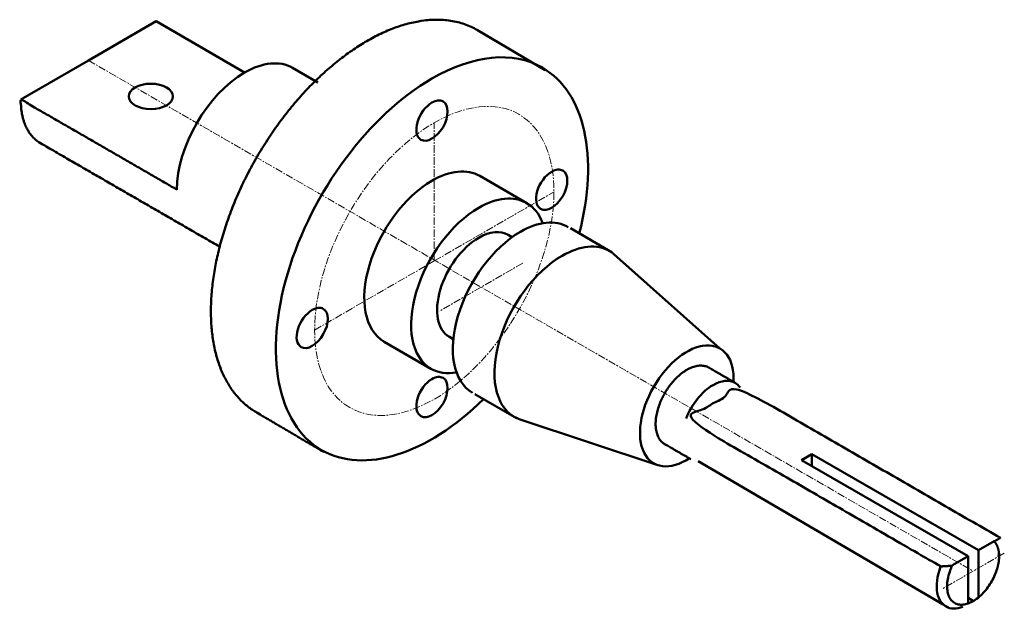
# Model space of a CAD drawing. Units: millimetres. Extents: x -23 to 141, y -9 to 89.
import ezdxf

# ---------------------------------------------------------------- set-up
doc = ezdxf.new("R2010")
doc.units = ezdxf.units.MM
doc.header["$MEASUREMENT"] = 0
doc.linetypes.add('CENTER', pattern=[2, 1.25, -0.25, 0.25, -0.25])
doc.layers.add('M-CNTR', color=4, linetype='CENTER', lineweight=18)
doc.layers.add('M-OUTL', color=7, linetype='Continuous', lineweight=50)

msp = doc.modelspace()

# ---------------------------------------------------------------- linework, layer by layer
at = {"layer": 'M-CNTR'}
for p, q in [((-11.24, 81.97), (135.98, -3.03)), ((46.33, 48.59), (46.33, 71.59)), ((61.05, 48.23), (47.19, 40.23)), ((141.18, -0.03), (130.79, -6.03))]:
    msp.add_line(p, q, dxfattribs=at)
msp.add_lwpolyline([(26.41, 37.09), (46.33, 48.59), (66.25, 60.09)], dxfattribs=at)
msp.add_ellipse((46.33, 48.59), major_axis=(-14.08, -24.4), ratio=0.57735, dxfattribs=at)
at = {"layer": 'M-OUTL'}
for p, q in [((53.5, 87.01), (64.8, 80.35)), ((26.95, 78.28), (22.72, 80.73)), ((61.7, 58.23), (53.9, 62.73)), ((59.29, 52.54), (58.63, 52.92)), ((69.01, 54.02), (75.94, 50.02)), ((75.72, 50.14), (93.86, 34.01)), ((45.77, 30.65), (37.98, 35.15)), ((49.49, 35.57), (48.84, 35.95)), ((53.09, 26.44), (60.02, 22.44)), ((83.55, 14.58), (60.62, 22.2)), ((109.16, 16.44), (107.43, 15.44)), ((136.87, 0.44), (109.16, 16.44)), ((109.16, 14.44), (109.16, 16.44)), ((90.25, 15.26), (131.02, -8.58)), ((135.14, -0.56), (107.43, 15.44)), ((136.87, 0.44), (139.47, 1.94)), ((136.87, 0.44), (136.87, -7.46)), ((132.54, -2.06), (135.14, -0.56)), ((135.14, -0.56), (135.14, -8.46)), ((136.01, -7.98), (135.14, -7.48))]:
    msp.add_line(p, q, dxfattribs=at)
msp.add_lwpolyline([(-22.5, 75.47), (-11.24, 81.97), (0.02, 88.47), (14.74, 79.97)], dxfattribs=at)
for centre, major_axis, start_param, end_param in [((45.94, 48.94), (18.37, 31.82), 0, 0.785398), ((14.76, 66.94), (7.96, 13.79), 0, 0.785398), ((45.94, 48.94), (18.37, 31.82), 5.160577, 6.283185), ((14.76, 66.94), (7.96, 13.79), 0.785398, 2.356194), ((45.94, 48.94), (18.37, 31.82), 0.785398, 3.141593), ((45.94, 71.94), (1.84, 3.18), 0, 0.785398), ((45.94, 71.94), (1.84, 3.18), 0.785398, 3.141593), ((45.94, 71.94), (1.84, 3.18), 3.141593, 6.283185), ((45.94, 48.94), (7.96, 13.79), 0, 0.785398), ((65.86, 60.44), (1.84, 3.18), 0, 0.785398), ((65.86, 60.44), (1.84, 3.18), 0.785398, 3.141593), ((65.86, 60.44), (1.84, 3.18), 3.141593, 6.283185), ((45.94, 48.94), (7.96, 13.79), 0.785398, 3.141593), ((53.73, 44.44), (7.96, 13.79), 0, 0.785398), ((53.73, 44.44), (7.96, 13.79), 0.785398, 3.141593), ((53.73, 44.44), (7.96, 13.79), 5.832989, 6.283185), ((60.66, 40.44), (7.96, 13.79), 0, 0.785398), ((53.73, 44.44), (4.9, 8.49), 0.785398, 3.141593), ((60.66, 40.44), (7.96, 13.79), 0.785398, 3.141593), ((53.73, 44.44), (4.9, 8.49), 0, 0.785398), ((67.59, 36.44), (7.96, 13.79), 0, 0.785398), ((67.59, 36.44), (7.96, 13.79), 0.785398, 3.141593), ((26.02, 37.44), (1.84, 3.18), 0.785398, 3.141593), ((26.02, 37.44), (1.84, 3.18), 3.141593, 6.283185), ((26.02, 37.44), (1.84, 3.18), 0, 0.785398), ((88.35, 24.47), (-5.51, -9.55), 2.298971, 7.125807), ((53.73, 44.44), (7.96, 13.79), 3.141593, 3.591789), ((45.94, 25.94), (1.84, 3.18), 0.785398, 3.141593), ((45.94, 25.94), (1.84, 3.18), 3.141593, 6.283185), ((45.94, 25.94), (1.84, 3.18), 0, 0.785398), ((92.71, 21.94), (3.67, 6.36), 0.785398, 1.832596), ((92.71, 21.94), (3.67, 6.36), 0, 0.785398), ((92.71, 21.94), (3.67, 6.36), 6.021386, 6.283185), ((45.94, 48.94), (18.37, 31.82), 3.141593, 4.264201), ((67.59, 36.44), (7.96, 13.79), 3.141593, 3.259718), ((135.12, -2.53), (-3.67, -6.36), 8.471932, 8.552132), ((135.12, -2.53), (-3.67, -6.36), 4.990265, 6.401311), ((135.14, -2.56), (3.67, 6.36), 3.141593, 3.759543)]:
    msp.add_ellipse(centre, major_axis=major_axis, ratio=0.57735, start_param=start_param, end_param=end_param, dxfattribs=at)
msp.add_ellipse((-0.85, 75.97), major_axis=(-3.67, 0), ratio=0.57735, dxfattribs=at)
for points, weights, knots in [([(53.69, 86.9), (43.16, 93.24), (28.58, 80.45), (14.01, 67.65), (10.06, 48.59), (6.11, 29.52), (16.76, 23.37), (22.36, 20.07), (27.96, 16.77)], [1, 0.865142408056, 1, 0.865142408056, 1, 0.865142408056, 1, 1, 1], [0, 0, 0, 1.050724, 1.050724, 2.101448, 2.101448, 3.152172, 3.152172, 4.152172, 4.152172, 4.152172]), ([(3.48, 60.47), (-9.51, 67.97), (-22.5, 75.47), (-22.5, 70.08), (-19.2, 68.18), (-4.29, 59.57), (10.61, 50.96)], [1, 1, 1, 0.923879532511, 1, 1, 1], [0, 0, 0, 1, 1, 1.785398, 1.785398, 2.785398, 2.785398, 2.785398]), ([(96.36, 28.33), (94.19, 29.58), (92.03, 30.83), (88.35, 32.95), (84.68, 26.59), (81, 20.22), (84.68, 18.1), (86.84, 16.85), (89.01, 15.6)], [1, 1, 1, 0.707106781187, 1, 0.707106781187, 1, 1, 1], [0, 0, 0, 1, 1, 2.570796, 2.570796, 4.141593, 4.141593, 5.141593, 5.141593, 5.141593]), ([(140.52, 2.5), (118.87, 15), (97.22, 27.5), (92.68, 24.88), (88.14, 22.26), (109.36, 10.01), (130.58, -2.24), (131.52, -2.19), (132.47, -2.15), (130.2, -7.1), (133.09, -8.42), (135.98, -9.75), (138.87, -5.09), (141.77, -0.42), (139.5, 1.91), (140.01, 2.21), (140.52, 2.5)], [1, 1, 1, 1, 1, 1, 1, 1, 1, 0.744400686611, 1, 0.744400686611, 1, 0.744400686611, 1, 1, 1], [0, 0, 0, 1, 1, 2, 2, 3, 3, 4, 4, 5.462319, 5.462319, 6.924638, 6.924638, 8.386957, 8.386957, 9.386957, 9.386957, 9.386957])]:
    msp.add_rational_spline(points, weights, degree=2, knots=knots, dxfattribs=at)

doc.saveas('drawing.dxf')
